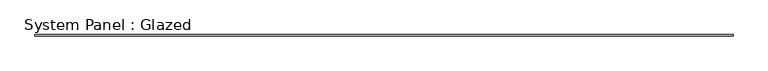
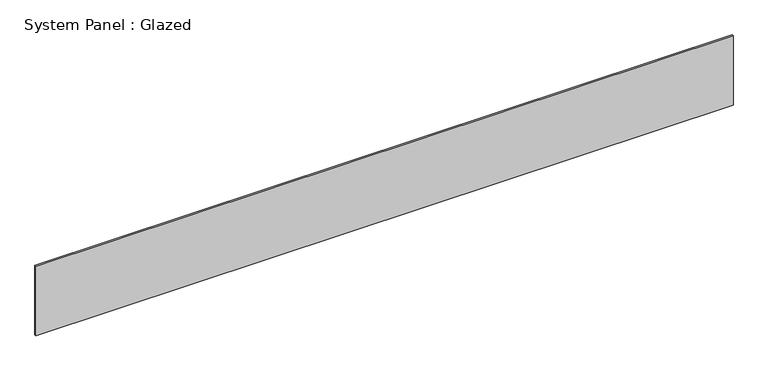
"""IFC4 building model written with IfcOpenShell, lengths in millimetres: plate geometry, System Panel : Glazed."""

from ifc_helpers import new_model, si_unit, origin, origin_with_axes, place, context, project, spatial, polyline, outline, extrude, source, transform, mapped, element, save


def system_panel_glazed_0853085d(model_context):
    return source(origin(), model_context, "Body", "SweptSolid", [
        extrude(outline(polyline([(5791.2, 19.05), (-5791.2, 19.05), (-5791.2, 44.45), (5791.2, 44.45), (5791.2, 19.05)])), origin_with_axes(), (0.0, 0.0, 1.0), 1219.2),
    ])


if __name__ == "__main__":
    model = new_model("IFC4")
    model_context = context("Model", 3, world=origin())
    ifc_project = project(units=[si_unit("LENGTHUNIT", "METRE", prefix="MILLI")], contexts=[model_context])
    site = spatial("IfcSite", under=ifc_project)
    building = spatial("IfcBuilding", under=site)
    placement = place(None, origin())
    system_panel_glazed_shape = system_panel_glazed_0853085d(model_context)
    element("IfcPlate", 1, ObjectType="System Panel : Glazed", at=placement, inside=building, context=model_context, shape_type="MappedRepresentation", body=[
        mapped(system_panel_glazed_shape, transform((0.0, 0.0, 0.0), x_axis=(1.0, 0.0, 0.0), y_axis=(0.0, 1.0, 0.0), z_axis=(0.0, 0.0, 1.0))),
    ])
    save(model, "model.ifc")

# Revit data of these elements
# Type "System Panel : Glazed"
#   Construction Type Id = "GSP4R"
#   Analytic Construction = "1/8 in Pilkington single glazing"
#   Visual Light Transmittance = 0.9
#   Solar Heat Gain Coefficient = 0.86
#   Heat Transfer Coefficient (U) = 1.18115 BTU/(h·ft²·°F)
# Element 1 (IfcPlate, "System Panel : Glazed")
#   Materials on its faces: "Glass"
# Materials
#   "Glass": class "Glass", colour RGB 0 128 192, transparency 0.75, Description = "Soda Lime Glass", Cost = 0
